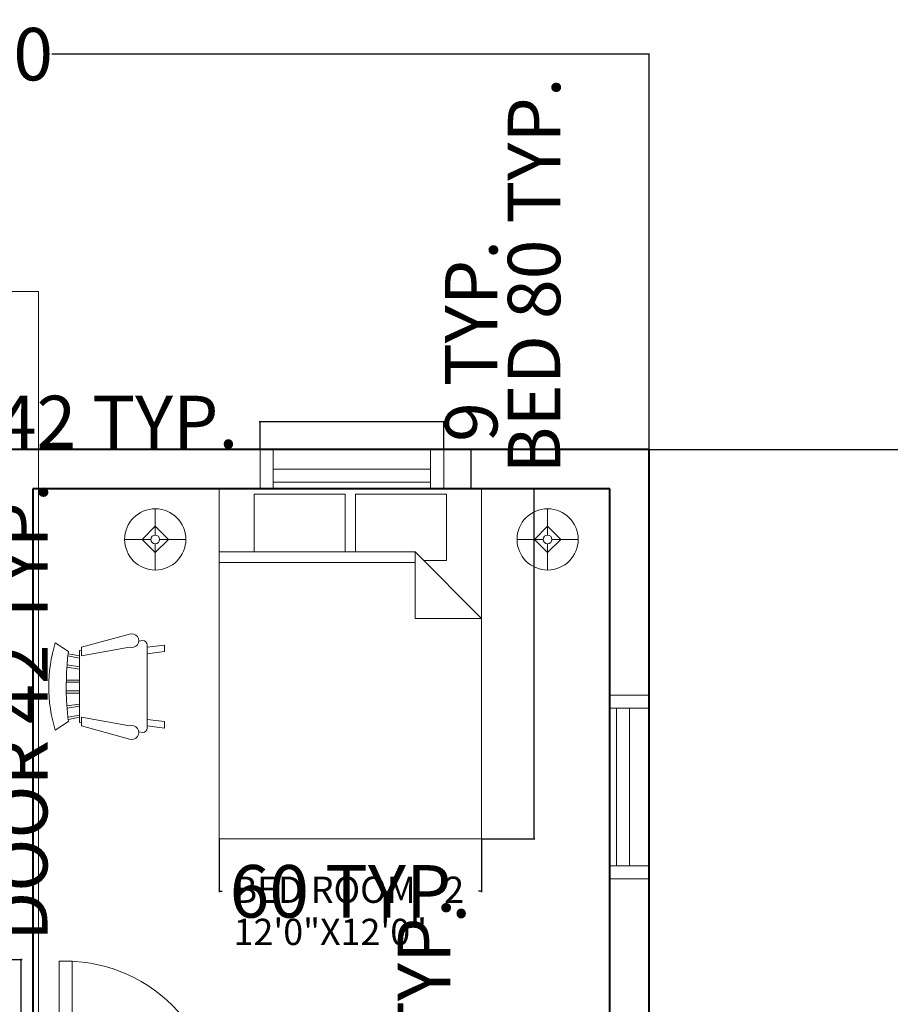
# Model space of a CAD drawing. Units: inches. Extents: x -101 to 786, y 26 to 880.
# Tile 5 of 9: x 180 to 379, y 655 to 880. Entities that reach past the tile are written whole.
import ezdxf

# ---------------------------------------------------------------- set-up
doc = ezdxf.new("R2010")
doc.units = ezdxf.units.IN
doc.header["$MEASUREMENT"] = 0
for name, color, linetype, lineweight in [('A-ANNO-DIMS', 2, 'Continuous', 18), ('A-ANNO-SYMB', 2, 'Continuous', 18), ('A-AREA-IDEN', 7, 'Continuous', 18), ('A-DOOR', 4, 'Continuous', 20), ('A-EQPM', 8, 'Continuous', 13), ('A-FURN', 8, 'Continuous', 13), ('A-GLAZ', 4, 'Continuous', 18), ('A-WALL', 7, 'Continuous', 40)]:
    doc.layers.add(name, color=color, linetype=linetype, lineweight=lineweight)
doc.styles.get("Standard").update_dxf_attribs({"font": 'arial.ttf'})
doc.dimstyles.get("Standard").update_dxf_attribs({"dimtxt": 12, "dimasz": 0.18, "dimexe": 0.18, "dimexo": 0.0625, "dimgap": 0.09, "dimtad": 0, "dimdec": 1, "dimzin": 0, "dimdsep": 46, "dimlunit": 3, "dimtxsty": 'Standard', "dimcen": 0.09, "dimadec": 0, "dimazin": 0, "dimtfac": 1, "dimtdec": 1, "dimtofl": 0, "dimtmove": 0, "dimatfit": 3, "dimfxl": 1, "dimtolj": 1, "dimtzin": 0, "dimarcsym": 0})

# ---------------------------------------------------------------- blocks, each defined once
blk = doc.blocks.new('Bed - Queen')
for p, q in [((0, -80.00003), (0, 0)), ((0, 0), (59.99999, 0)), ((59.99999, 0), (59.99999, -80.00003)), ((7.99999, -1.2), (28.79998, -1.2)), ((7.99999, -14.4), (7.99999, -1.2)), ((28.79998, -1.2), (28.79998, -14.4)), ((31.19999, -1.2), (51.99999, -1.2)), ((31.19999, -14.4), (31.19999, -1.2)), ((51.99999, -1.2), (51.99999, -16.4)), ((0, -14.4), (44.8, -14.4)), ((59.99999, -29.6), (44.8, -14.4)), ((44.8, -14.4), (44.8, -29.6)), ((44.8, -16.8), (0, -16.8)), ((51.99999, -16.4), (46.79936, -16.4)), ((44.8, -29.6), (59.99999, -29.6)), ((59.99999, -80.00003), (0, -80.00003))]:
    blk.add_line(p, q)
blk = doc.blocks.new('Lamp - Table')
for p, q in [((0, 7), (0, 1)), ((0, 3), (-3, 0)), ((3, 0), (0, 3)), ((-1, 0), (-7, 0)), ((-3, 0), (0, -3)), ((0, -3), (3, 0)), ((1, 0), (7, 0)), ((0, -1), (0, -7))]:
    blk.add_line(p, q)
for radius in [7, 1]:
    blk.add_circle((0, 0), radius)
blk = doc.blocks.new('Chair - Rocking')
for p, q in [((-8, -4.5), (-10, -1.5)), ((8, -4.5), (10, -1.5)), ((-7.5, -4.5), (-7, -7)), ((-6.5, -7), (-7.02225, -4.43)), ((-4.5, -7), (-4.96674, -4.19951)), ((-4, -7), (-4.40532, -4.16272)), ((-1.5, -4.05012), (-1.5, -7)), ((-1, -7), (-1, -4.05012)), ((1, -7), (1, -4.04655)), ((1.5, -4.05012), (1.5, -7)), ((4, -7), (4.40187, -4.18694)), ((4.5, -7), (4.96761, -4.19437)), ((6.5, -7), (7, -4.4057)), ((7.5, -4.5), (7, -7)), ((-9, -7.5), (-12, -18.49999)), ((-7, -7.5), (-9, -7.5)), ((-9, -18.49999), (-7, -7.5)), ((-8.23428, -6.99939), (-8.3093, -7.47958)), ((-8.23041, -7), (8.23915, -7)), ((7, -7.5), (9, -7.5)), ((9, -18.49999), (7, -7.5)), ((8.31071, -7.48854), (8.23449, -7.00073)), ((9, -7.5), (12, -18.49999)), ((-10.36644, -20.64523), (-10.5, -21.49999)), ((-9, -22.49999), (-9.5, -26.49999)), ((0, -22.49999), (-9.5, -22.49999)), ((-8, -26.49999), (-7.5, -22.49999)), ((0, -22.49999), (9.5, -22.49999)), ((8, -26.49999), (7.5, -22.49999)), ((9, -22.49999), (9.5, -26.49999)), ((10.5, -21.49999), (10.3575, -20.58798)), ((-9.5, -26.49999), (-8, -26.49999)), ((9.5, -26.49999), (8, -26.49999))]:
    blk.add_line(p, q)
for centre, radius, start, end in [((0, -34.08333), 34.08333, 72.93847, 107.0615), ((0, -68.25004), 64.25, 93.92211, 97.15267), ((0, -68.25004), 64.25, 82.84733, 93.92211), ((-10.5, -18.99999), 1.58114, 161.5651, 18.43495), ((10.5, -18.99999), 1.58114, 161.5651, 18.43495), ((-9.5, -21.49999), 1, 180, 270), ((9.5, -21.49999), 1, 270, 0)]:
    blk.add_arc(centre, radius, start, end)
blk = doc.blocks.new('DOOR-SINGLE-36')
for p, q in [((-39, 0), (-39, -6)), ((-36, 0), (-36, -6)), ((0, 0), (0, -6)), ((3, 0), (3, -6))]:
    blk.add_line(p, q)
blk.add_lwpolyline([(0, 0), (-3, 0), (-3, 36), (0, 36)], close=True)
blk.add_arc((-1.5, 1.5), 34.53, 87.5104, 182.4896)
blk = doc.blocks.new('WIN-36-WALL9')
for p, q in [((0, 42), (9, 42)), ((0, 39), (9, 39)), ((1.5, 39), (1.5, 3)), ((4.5, 39), (4.5, 3)), ((9, 3), (0, 3)), ((9, 0), (0, 0))]:
    blk.add_line(p, q)
blk = doc.blocks.new('*D35')
at = {"layer": 'A-ANNO-DIMS', "color": 0, "lineweight": -2, "transparency": 16777216}
for p, q in [((173.57, 665.22), (180.05, 665.22)), ((179.87, 665.22), (179.87, 665.4)), ((179.87, 622.98), (179.87, 665.04)), ((173.57, 622.8), (180.05, 622.8))]:
    blk.add_line(p, q, dxfattribs=at)
at = {"layer": 'A-ANNO-DIMS', "color": 0, "transparency": 16777216}
for points in [[(179.84, 665.04), (179.9, 665.04), (179.87, 665.22)], [(179.84, 622.98), (179.9, 622.98), (179.87, 622.8)]]:
    blk.add_solid(points, dxfattribs=at)
at = {"layer": 'Defpoints', "color": 0, "transparency": 16777216}
for p in [(173.51, 665.22), (179.87, 665.22), (173.51, 622.8)]:
    blk.add_point(p, dxfattribs=at)
at = {"layer": 'A-ANNO-DIMS', "color": 0, "transparency": 16777216, "insert": (179.87, 721.88), "char_height": 12, "attachment_point": 5, "rotation": 90}
blk.add_mtext('\\A1;DOOR 42 TYP.', dxfattribs=at)
blk = doc.blocks.new('*D37')
at = {"layer": 'A-ANNO-DIMS', "color": 0, "lineweight": -2, "transparency": 16777216}
for p, q in [((234.49, 788.1), (234.31, 788.1)), ((234.49, 781.87), (234.49, 788.28)), ((276.31, 788.1), (234.67, 788.1)), ((276.49, 781.87), (276.49, 788.28))]:
    blk.add_line(p, q, dxfattribs=at)
at = {"layer": 'A-ANNO-DIMS', "color": 0, "transparency": 16777216}
for points in [[(234.67, 788.13), (234.67, 788.07), (234.49, 788.1)], [(276.31, 788.13), (276.31, 788.07), (276.49, 788.1)]]:
    blk.add_solid(points, dxfattribs=at)
at = {"layer": 'Defpoints', "color": 0, "transparency": 16777216}
for p in [(234.49, 788.1), (234.49, 781.8), (276.49, 781.8)]:
    blk.add_point(p, dxfattribs=at)
at = {"layer": 'A-ANNO-DIMS', "color": 0, "transparency": 16777216, "insert": (165.66, 788.1), "char_height": 12, "attachment_point": 5}
blk.add_mtext('\\A1;WINDOW 42 TYP.', dxfattribs=at)
blk = doc.blocks.new('*D38')
at = {"layer": 'A-ANNO-DIMS', "color": 0, "lineweight": -2, "transparency": 16777216}
for p, q in [((276.55, 781.8), (282.97, 781.8)), ((282.79, 781.8), (282.79, 781.98)), ((282.79, 772.98), (282.79, 781.62)), ((276.55, 772.8), (282.97, 772.8))]:
    blk.add_line(p, q, dxfattribs=at)
at = {"layer": 'A-ANNO-DIMS', "color": 0, "transparency": 16777216}
for points in [[(282.76, 781.62), (282.82, 781.62), (282.79, 781.8)], [(282.76, 772.98), (282.82, 772.98), (282.79, 772.8)]]:
    blk.add_solid(points, dxfattribs=at)
at = {"layer": 'Defpoints', "color": 0, "transparency": 16777216}
for p in [(276.49, 781.8), (282.79, 781.8), (276.49, 772.8)]:
    blk.add_point(p, dxfattribs=at)
at = {"layer": 'A-ANNO-DIMS', "color": 0, "transparency": 16777216, "insert": (282.79, 806.62), "char_height": 12, "attachment_point": 5, "rotation": 90}
blk.add_mtext('\\A1;9 TYP.', dxfattribs=at)
blk = doc.blocks.new('*D44')
at = {"layer": 'A-ANNO-DIMS', "color": 0, "lineweight": -2, "transparency": 16777216}
for p, q in [((269.02, 622.8), (272.15, 622.8)), ((271.97, 622.8), (271.97, 622.98)), ((271.97, 609.59), (271.97, 622.62)), ((269.02, 609.41), (272.15, 609.41))]:
    blk.add_line(p, q, dxfattribs=at)
at = {"layer": 'A-ANNO-DIMS', "color": 0, "transparency": 16777216}
for points in [[(271.94, 622.62), (272, 622.62), (271.97, 622.8)], [(271.94, 609.59), (272, 609.59), (271.97, 609.41)]]:
    blk.add_solid(points, dxfattribs=at)
at = {"layer": 'Defpoints', "color": 0, "transparency": 16777216}
for p in [(268.95, 622.8), (271.97, 622.8), (268.95, 609.41)]:
    blk.add_point(p, dxfattribs=at)
at = {"layer": 'A-ANNO-DIMS', "color": 0, "transparency": 16777216, "insert": (271.97, 651.71), "char_height": 12, "attachment_point": 5, "rotation": 90}
blk.add_mtext('\\A1;13 TYP.', dxfattribs=at)
blk = doc.blocks.new('*D47')
at = {"layer": 'A-ANNO-DIMS', "color": 0, "lineweight": -2, "transparency": 16777216}
for p, q in [((285.21, 772.8), (297.32, 772.8)), ((297.14, 772.8), (297.14, 772.98)), ((297.14, 692.98), (297.14, 772.62)), ((285.21, 692.8), (297.32, 692.8))]:
    blk.add_line(p, q, dxfattribs=at)
at = {"layer": 'A-ANNO-DIMS', "color": 0, "transparency": 16777216}
for points in [[(297.11, 772.62), (297.17, 772.62), (297.14, 772.8)], [(297.11, 692.98), (297.17, 692.98), (297.14, 692.8)]]:
    blk.add_solid(points, dxfattribs=at)
at = {"layer": 'Defpoints', "color": 0, "transparency": 16777216}
for p in [(285.14, 772.8), (297.14, 772.8), (285.14, 692.8)]:
    blk.add_point(p, dxfattribs=at)
at = {"layer": 'A-ANNO-DIMS', "color": 0, "transparency": 16777216, "insert": (297.14, 821.58), "char_height": 12, "attachment_point": 5, "rotation": 90}
blk.add_mtext('\\A1;BED 80 TYP.', dxfattribs=at)
blk = doc.blocks.new('*D48')
at = {"layer": 'A-ANNO-DIMS', "color": 0, "lineweight": -2, "transparency": 16777216}
for p, q in [((225.14, 692.74), (225.14, 680.62)), ((285.14, 692.74), (285.14, 680.62)), ((225.32, 680.8), (225.82, 680.8)), ((284.96, 680.8), (284.47, 680.8))]:
    blk.add_line(p, q, dxfattribs=at)
at = {"layer": 'A-ANNO-DIMS', "color": 0, "transparency": 16777216}
for points in [[(225.32, 680.83), (225.32, 680.77), (225.14, 680.8)], [(284.96, 680.83), (284.96, 680.77), (285.14, 680.8)]]:
    blk.add_solid(points, dxfattribs=at)
at = {"layer": 'Defpoints', "color": 0, "transparency": 16777216}
for p in [(225.14, 692.8), (285.14, 692.8), (285.14, 680.8)]:
    blk.add_point(p, dxfattribs=at)
at = {"layer": 'A-ANNO-DIMS', "color": 0, "transparency": 16777216, "insert": (255.14, 680.8), "char_height": 12, "attachment_point": 5}
blk.add_mtext('\\A1;60 TYP.', dxfattribs=at)
blk = doc.blocks.new('*D79')
at = {"layer": 'A-ANNO-DIMS', "color": 0, "lineweight": -2, "transparency": 16777216}
for p, q in [((23.51, 781.87), (23.51, 872.36)), ((23.69, 872.18), (160.19, 872.18)), ((323.33, 872.18), (186.83, 872.18)), ((323.51, 781.87), (323.51, 872.36))]:
    blk.add_line(p, q, dxfattribs=at)
at = {"layer": 'A-ANNO-DIMS', "color": 0, "transparency": 16777216}
for points in [[(23.69, 872.21), (23.69, 872.15), (23.51, 872.18)], [(323.33, 872.21), (323.33, 872.15), (323.51, 872.18)]]:
    blk.add_solid(points, dxfattribs=at)
at = {"layer": 'Defpoints', "color": 0, "transparency": 16777216}
for p in [(323.51, 872.18), (23.51, 781.8), (323.51, 781.8)]:
    blk.add_point(p, dxfattribs=at)
at = {"layer": 'A-ANNO-DIMS', "color": 0, "transparency": 16777216, "insert": (173.51, 872.18), "char_height": 12, "attachment_point": 5}
blk.add_mtext('\\A1;300', dxfattribs=at)
blk = doc.blocks.new('*D80')
at = {"layer": 'A-ANNO-DIMS', "color": 0, "lineweight": -2, "transparency": 16777216}
for p, q in [((323.57, 781.8), (424.94, 781.8)), ((424.76, 781.62), (424.76, 472.49)), ((424.76, 122.52), (424.76, 431.66)), ((323.57, 122.34), (424.94, 122.34))]:
    blk.add_line(p, q, dxfattribs=at)
at = {"layer": 'A-ANNO-DIMS', "color": 0, "transparency": 16777216}
for points in [[(424.73, 781.62), (424.79, 781.62), (424.76, 781.8)], [(424.73, 122.52), (424.79, 122.52), (424.76, 122.34)]]:
    blk.add_solid(points, dxfattribs=at)
at = {"layer": 'Defpoints', "color": 0, "transparency": 16777216}
for p in [(323.51, 781.8), (424.76, 781.8), (323.51, 122.34)]:
    blk.add_point(p, dxfattribs=at)
at = {"layer": 'A-ANNO-DIMS', "color": 0, "transparency": 16777216, "insert": (424.76, 452.07), "char_height": 12, "attachment_point": 5, "rotation": 90}
blk.add_mtext('\\A1;659.5', dxfattribs=at)

msp = doc.modelspace()

# ---------------------------------------------------------------- linework, layer by layer
at = {"layer": 'A-ANNO-SYMB'}
for p, q in [((183.8117, 817.9238), (157.8207, 817.9238)), ((183.8117, 802.4238), (183.8117, 817.9238)), ((183.8117, 802.4238), (183.8117, 309.6043))]:
    msp.add_line(p, q, dxfattribs=at)
at = {"layer": 'A-WALL'}
for p, q in [((314.5071, 772.8033), (182.5071, 772.8033)), ((182.5071, 772.8033), (182.5071, 628.8033)), ((314.5071, 628.8033), (314.5071, 772.8033))]:
    msp.add_line(p, q, dxfattribs=at)
msp.add_lwpolyline([(323.5071, 151.8033), (323.5071, 781.8033), (23.5071, 781.8033), (23.5071, 151.8033)], dxfattribs=at)

# ---------------------------------------------------------------- block references
at = {"layer": 'A-DOOR', "extrusion": (0, 0, -1), "zscale": -1}
msp.add_blockref('DOOR-SINGLE-36', (-188.5071, 628.8033), dxfattribs=at)
at = {"layer": 'A-EQPM'}
for p in [(210.5116, 761.25), (300.2532, 761.25)]:
    msp.add_blockref('Lamp - Table', p, dxfattribs=at)
at = {"layer": 'A-FURN'}
msp.add_blockref('Bed - Queen', (225.1445, 772.8033), dxfattribs=at)
at = {"layer": 'A-FURN', "rotation": 90}
msp.add_blockref('Chair - Rocking', (186.1516, 727.6063), dxfattribs=at)
at = {"layer": 'A-GLAZ', "rotation": 89.99999999999994}
msp.add_blockref('WIN-36-WALL9', (276.4852, 772.8032), dxfattribs=at)
at = {"layer": 'A-GLAZ'}
msp.add_blockref('WIN-36-WALL9', (314.507, 683.6419), dxfattribs=at)

# ---------------------------------------------------------------- texts
at = {"layer": 'A-AREA-IDEN'}
for s, p in [('BED ROOM - 2', (228.433, 678.1607)), ('12\'0"X12\'0"', (228.433, 668.5222))]:
    msp.add_text(s, height=6, dxfattribs=at).set_placement(p)

# ---------------------------------------------------------------- dimensions: what is measured, and where the dimension line sits
at = {"layer": 'A-ANNO-DIMS'}
dim = msp.add_linear_dim(base=(323.5071, 872.1827), p1=(23.5071, 781.8033), p2=(323.5071, 781.8033), dimstyle='Standard', override={"dimdec": 0, "dimlfac": 1, "dimrnd": 0, "dimzin": 0, "dimdsep": 46, "dimlunit": 2}, dxfattribs=at)
dim.commit()
dim.dimension.update_dxf_attribs({"geometry": '*D79', "text_midpoint": (173.5071, 872.1827)})
for base, p1, p2, angle, text, picture, middle in [((297.1445, 772.8033), (285.1445, 692.8033), (285.1445, 772.8033), 90, 'BED <> TYP.', '*D47', (297.1445, 821.5767)), ((282.7852, 781.8033), (276.4852, 772.8033), (276.4852, 781.8033), 90, '<> TYP.', '*D38', (282.7852, 806.6176)), ((234.4852, 788.1033), (276.4852, 781.8033), (234.4852, 781.8033), 180, 'WINDOW <> TYP.', '*D37', (165.6572, 788.1033)), ((179.8701, 665.2238), (173.5071, 622.8033), (173.5071, 665.2238), 90, 'DOOR <> TYP.', '*D35', (179.8701, 721.8757)), ((271.9694, 622.8033), (268.9548, 609.4053), (268.9548, 622.8033), 90, '<> TYP.', '*D44', (271.9694, 651.7145))]:
    dim = msp.add_linear_dim(base=base, p1=p1, p2=p2, angle=angle, text=text, dimstyle='Standard', override={"dimdec": 0, "dimlfac": 1, "dimrnd": 0, "dimzin": 0, "dimdsep": 46, "dimlunit": 2}, dxfattribs=at)
    dim.commit()
    dim.dimension.update_dxf_attribs({"geometry": picture, "text_midpoint": middle})
dim = msp.add_linear_dim(base=(424.7579, 781.8033), p1=(323.5071, 122.3446), p2=(323.5071, 781.8033), angle=90, dimstyle='Standard', override={"dimdec": 1, "dimlfac": 1, "dimrnd": 0, "dimzin": 0, "dimdsep": 46, "dimlunit": 2}, dxfattribs=at)
dim.commit()
dim.dimension.update_dxf_attribs({"geometry": '*D80', "text_midpoint": (424.7579, 452.0739)})
dim = msp.add_linear_dim(base=(285.1445, 680.8033), p1=(225.1445, 692.8033), p2=(285.1445, 692.8033), text='<> TYP.', dimstyle='Standard', override={"dimdec": 0, "dimlfac": 1, "dimrnd": 0, "dimzin": 0, "dimdsep": 46, "dimlunit": 2}, dxfattribs=at)
dim.commit()
dim.dimension.update_dxf_attribs({"geometry": '*D48', "text_midpoint": (255.1445, 680.8033)})

doc.saveas('drawing.dxf')
